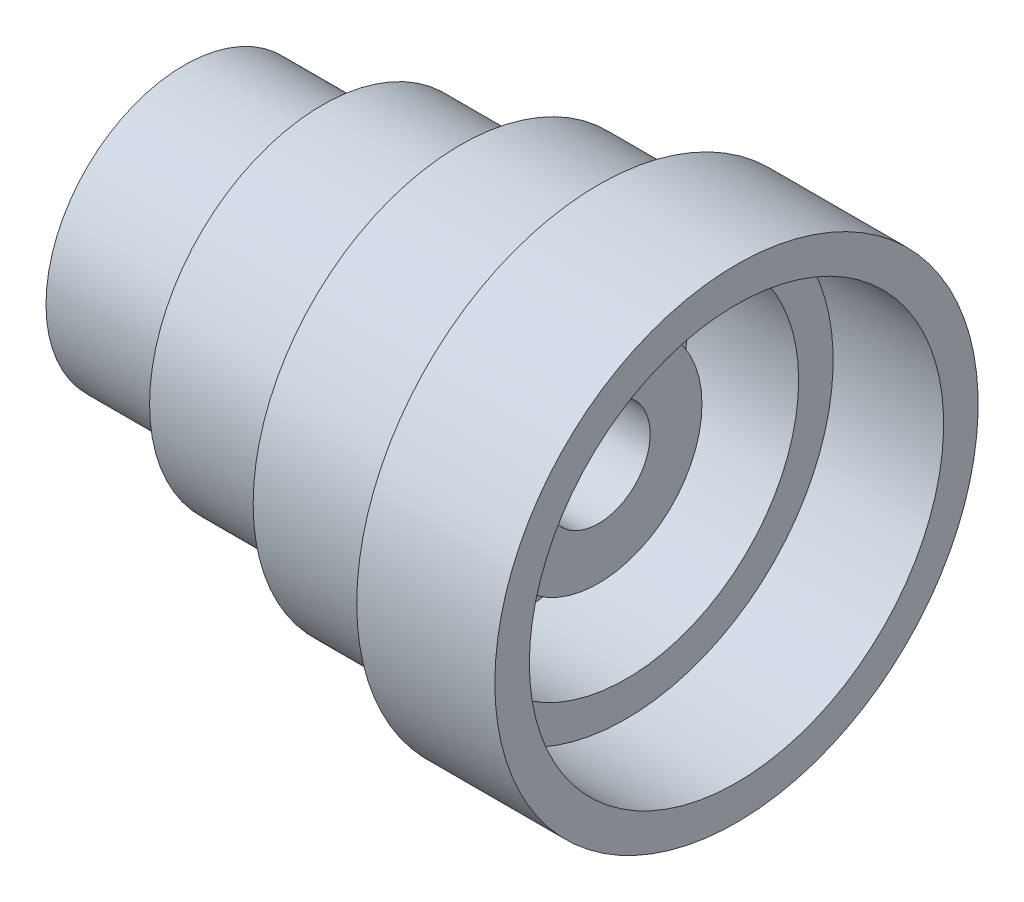
ISO-10303-21;
HEADER;
FILE_DESCRIPTION(('STEP AP214'),'2;1');
FILE_NAME('part.step','',(''),(''),'','','');
FILE_SCHEMA(('AUTOMOTIVE_DESIGN { 1 0 10303 214 1 1 1 1 }'));
ENDSEC;
DATA;
#1=APPLICATION_CONTEXT('core data for automotive mechanical design processes');
#2=APPLICATION_PROTOCOL_DEFINITION('international standard','automotive_design',2000,#1);
#3=PRODUCT_CONTEXT('',#1,'mechanical');
#4=PRODUCT('Part','Part','',(#3));
#5=PRODUCT_RELATED_PRODUCT_CATEGORY('part','',(#4));
#6=PRODUCT_DEFINITION_FORMATION('','',#4);
#7=PRODUCT_DEFINITION_CONTEXT('part definition',#1,'design');
#8=PRODUCT_DEFINITION('design','',#6,#7);
#9=PRODUCT_DEFINITION_SHAPE('','',#8);
#10=(LENGTH_UNIT() NAMED_UNIT(*) SI_UNIT(.MILLI.,.METRE.));
#11=(NAMED_UNIT(*) PLANE_ANGLE_UNIT() SI_UNIT($,.RADIAN.));
#12=(NAMED_UNIT(*) SI_UNIT($,.STERADIAN.) SOLID_ANGLE_UNIT());
#13=UNCERTAINTY_MEASURE_WITH_UNIT(LENGTH_MEASURE(1.E-05),#10,'distance_accuracy_value','');
#14=(GEOMETRIC_REPRESENTATION_CONTEXT(3) GLOBAL_UNCERTAINTY_ASSIGNED_CONTEXT((#13)) GLOBAL_UNIT_ASSIGNED_CONTEXT((#10,
#11,#12)) REPRESENTATION_CONTEXT('',''));
#15=CARTESIAN_POINT('',(0.,0.,0.));
#16=DIRECTION('',(0.,0.,1.));
#17=DIRECTION('',(1.,0.,0.));
#18=AXIS2_PLACEMENT_3D('',#15,#16,#17);
#19=CARTESIAN_POINT('',(-96.9856636191065,0.,0.));
#20=DIRECTION('',(-1.,0.,0.));
#21=DIRECTION('',(0.,0.,1.));
#22=AXIS2_PLACEMENT_3D('',#19,#20,#21);
#23=CYLINDRICAL_SURFACE('',#22,15.);
#24=CARTESIAN_POINT('',(77.592099478672,0.,0.));
#25=DIRECTION('',(-1.,0.,0.));
#26=DIRECTION('',(0.,0.,1.));
#27=AXIS2_PLACEMENT_3D('',#24,#25,#26);
#28=CIRCLE('',#27,15.);
#29=CARTESIAN_POINT('',(77.592099478672,0.,15.));
#30=VERTEX_POINT('',#29);
#31=EDGE_CURVE('E10',#30,#30,#28,.T.);
#32=ORIENTED_EDGE('',*,*,#31,.F.);
#33=EDGE_LOOP('',(#32));
#34=FACE_BOUND('',#33,.T.);
#35=CARTESIAN_POINT('',(-42.407900521328,0.,0.));
#36=DIRECTION('',(-1.,0.,0.));
#37=DIRECTION('',(0.,0.,1.));
#38=AXIS2_PLACEMENT_3D('',#35,#36,#37);
#39=CIRCLE('',#38,15.);
#40=CARTESIAN_POINT('',(-42.407900521328,0.,15.));
#41=VERTEX_POINT('',#40);
#42=EDGE_CURVE('E92',#41,#41,#39,.T.);
#43=ORIENTED_EDGE('',*,*,#42,.T.);
#44=EDGE_LOOP('',(#43));
#45=FACE_BOUND('',#44,.T.);
#46=ADVANCED_FACE('F40',(#34,#45),#23,.F.);
#47=CARTESIAN_POINT('',(77.592099478672,15.,0.));
#48=DIRECTION('',(-1.,0.,0.));
#49=DIRECTION('',(0.,0.,1.));
#50=AXIS2_PLACEMENT_3D('',#47,#48,#49);
#51=PLANE('',#50);
#52=CARTESIAN_POINT('',(77.592099478672,0.,0.));
#53=DIRECTION('',(-1.,0.,0.));
#54=DIRECTION('',(0.,0.,1.));
#55=AXIS2_PLACEMENT_3D('',#52,#53,#54);
#56=CIRCLE('',#55,30.);
#57=CARTESIAN_POINT('',(77.592099478672,0.,30.));
#58=VERTEX_POINT('',#57);
#59=EDGE_CURVE('E43',#58,#58,#56,.T.);
#60=ORIENTED_EDGE('',*,*,#59,.F.);
#61=EDGE_LOOP('',(#60));
#62=FACE_BOUND('',#61,.T.);
#63=ORIENTED_EDGE('',*,*,#31,.T.);
#64=EDGE_LOOP('',(#63));
#65=FACE_BOUND('',#64,.T.);
#66=ADVANCED_FACE('F195',(#62,#65),#51,.F.);
#67=CARTESIAN_POINT('',(-96.9856636191065,0.,0.));
#68=DIRECTION('',(-1.,0.,0.));
#69=DIRECTION('',(0.,0.,1.));
#70=AXIS2_PLACEMENT_3D('',#67,#68,#69);
#71=CYLINDRICAL_SURFACE('',#70,30.);
#72=CARTESIAN_POINT('',(21.592099478672,0.,0.));
#73=DIRECTION('',(-1.,0.,0.));
#74=DIRECTION('',(0.,0.,1.));
#75=AXIS2_PLACEMENT_3D('',#72,#73,#74);
#76=CIRCLE('',#75,30.);
#77=CARTESIAN_POINT('',(21.592099478672,0.,30.));
#78=VERTEX_POINT('',#77);
#79=EDGE_CURVE('E50',#78,#78,#76,.T.);
#80=ORIENTED_EDGE('',*,*,#79,.F.);
#81=EDGE_LOOP('',(#80));
#82=FACE_BOUND('',#81,.T.);
#83=ORIENTED_EDGE('',*,*,#59,.T.);
#84=EDGE_LOOP('',(#83));
#85=FACE_BOUND('',#84,.T.);
#86=ADVANCED_FACE('F190',(#82,#85),#71,.T.);
#87=CARTESIAN_POINT('',(21.592099478672,40.,0.));
#88=DIRECTION('',(-1.,0.,0.));
#89=DIRECTION('',(0.,0.,1.));
#90=AXIS2_PLACEMENT_3D('',#87,#88,#89);
#91=PLANE('',#90);
#92=CARTESIAN_POINT('',(21.592099478672,0.,0.));
#93=DIRECTION('',(-1.,0.,0.));
#94=DIRECTION('',(0.,0.,1.));
#95=AXIS2_PLACEMENT_3D('',#92,#93,#94);
#96=CIRCLE('',#95,40.);
#97=CARTESIAN_POINT('',(21.592099478672,0.,40.));
#98=VERTEX_POINT('',#97);
#99=EDGE_CURVE('E51',#98,#98,#96,.T.);
#100=ORIENTED_EDGE('',*,*,#99,.F.);
#101=EDGE_LOOP('',(#100));
#102=FACE_BOUND('',#101,.T.);
#103=ORIENTED_EDGE('',*,*,#79,.T.);
#104=EDGE_LOOP('',(#103));
#105=FACE_BOUND('',#104,.T.);
#106=ADVANCED_FACE('F182',(#102,#105),#91,.F.);
#107=CARTESIAN_POINT('',(-96.9856636191065,0.,0.));
#108=DIRECTION('',(-1.,0.,0.));
#109=DIRECTION('',(0.,0.,1.));
#110=AXIS2_PLACEMENT_3D('',#107,#108,#109);
#111=CYLINDRICAL_SURFACE('',#110,40.);
#112=CARTESIAN_POINT('',(53.592099478672,0.,0.));
#113=DIRECTION('',(-1.,0.,0.));
#114=DIRECTION('',(0.,0.,1.));
#115=AXIS2_PLACEMENT_3D('',#112,#113,#114);
#116=CIRCLE('',#115,40.);
#117=CARTESIAN_POINT('',(53.592099478672,0.,40.));
#118=VERTEX_POINT('',#117);
#119=EDGE_CURVE('E57',#118,#118,#116,.T.);
#120=ORIENTED_EDGE('',*,*,#119,.F.);
#121=EDGE_LOOP('',(#120));
#122=FACE_BOUND('',#121,.T.);
#123=ORIENTED_EDGE('',*,*,#99,.T.);
#124=EDGE_LOOP('',(#123));
#125=FACE_BOUND('',#124,.T.);
#126=ADVANCED_FACE('F173',(#122,#125),#111,.F.);
#127=CARTESIAN_POINT('',(53.592099478672,50.,0.));
#128=DIRECTION('',(-1.,0.,0.));
#129=DIRECTION('',(0.,0.,1.));
#130=AXIS2_PLACEMENT_3D('',#127,#128,#129);
#131=PLANE('',#130);
#132=CARTESIAN_POINT('',(53.592099478672,0.,0.));
#133=DIRECTION('',(-1.,0.,0.));
#134=DIRECTION('',(0.,0.,1.));
#135=AXIS2_PLACEMENT_3D('',#132,#133,#134);
#136=CIRCLE('',#135,50.);
#137=CARTESIAN_POINT('',(53.592099478672,0.,50.));
#138=VERTEX_POINT('',#137);
#139=EDGE_CURVE('E56',#138,#138,#136,.T.);
#140=ORIENTED_EDGE('',*,*,#139,.F.);
#141=EDGE_LOOP('',(#140));
#142=FACE_BOUND('',#141,.T.);
#143=ORIENTED_EDGE('',*,*,#119,.T.);
#144=EDGE_LOOP('',(#143));
#145=FACE_BOUND('',#144,.T.);
#146=ADVANCED_FACE('F166',(#142,#145),#131,.F.);
#147=CARTESIAN_POINT('',(-96.9856636191065,0.,0.));
#148=DIRECTION('',(-1.,0.,0.));
#149=DIRECTION('',(0.,0.,1.));
#150=AXIS2_PLACEMENT_3D('',#147,#148,#149);
#151=CYLINDRICAL_SURFACE('',#150,50.);
#152=CARTESIAN_POINT('',(85.592099478672,0.,0.));
#153=DIRECTION('',(-1.,0.,0.));
#154=DIRECTION('',(0.,0.,1.));
#155=AXIS2_PLACEMENT_3D('',#152,#153,#154);
#156=CIRCLE('',#155,50.);
#157=CARTESIAN_POINT('',(85.592099478672,0.,50.));
#158=VERTEX_POINT('',#157);
#159=EDGE_CURVE('E65',#158,#158,#156,.T.);
#160=ORIENTED_EDGE('',*,*,#159,.F.);
#161=EDGE_LOOP('',(#160));
#162=FACE_BOUND('',#161,.T.);
#163=ORIENTED_EDGE('',*,*,#139,.T.);
#164=EDGE_LOOP('',(#163));
#165=FACE_BOUND('',#164,.T.);
#166=ADVANCED_FACE('F162',(#162,#165),#151,.F.);
#167=CARTESIAN_POINT('',(85.592099478672,60.,0.));
#168=DIRECTION('',(-1.,0.,0.));
#169=DIRECTION('',(0.,0.,1.));
#170=AXIS2_PLACEMENT_3D('',#167,#168,#169);
#171=PLANE('',#170);
#172=CARTESIAN_POINT('',(85.592099478672,0.,0.));
#173=DIRECTION('',(-1.,0.,0.));
#174=DIRECTION('',(0.,0.,1.));
#175=AXIS2_PLACEMENT_3D('',#172,#173,#174);
#176=CIRCLE('',#175,60.);
#177=CARTESIAN_POINT('',(85.592099478672,0.,60.));
#178=VERTEX_POINT('',#177);
#179=EDGE_CURVE('E63',#178,#178,#176,.T.);
#180=ORIENTED_EDGE('',*,*,#179,.F.);
#181=EDGE_LOOP('',(#180));
#182=FACE_BOUND('',#181,.T.);
#183=ORIENTED_EDGE('',*,*,#159,.T.);
#184=EDGE_LOOP('',(#183));
#185=FACE_BOUND('',#184,.T.);
#186=ADVANCED_FACE('F160',(#182,#185),#171,.F.);
#187=CARTESIAN_POINT('',(-96.9856636191065,0.,0.));
#188=DIRECTION('',(-1.,0.,0.));
#189=DIRECTION('',(0.,0.,1.));
#190=AXIS2_PLACEMENT_3D('',#187,#188,#189);
#191=CYLINDRICAL_SURFACE('',#190,60.);
#192=CARTESIAN_POINT('',(117.592099478672,0.,0.));
#193=DIRECTION('',(-1.,0.,0.));
#194=DIRECTION('',(0.,0.,1.));
#195=AXIS2_PLACEMENT_3D('',#192,#193,#194);
#196=CIRCLE('',#195,60.);
#197=CARTESIAN_POINT('',(117.592099478672,0.,60.));
#198=VERTEX_POINT('',#197);
#199=EDGE_CURVE('E67',#198,#198,#196,.T.);
#200=ORIENTED_EDGE('',*,*,#199,.F.);
#201=EDGE_LOOP('',(#200));
#202=FACE_BOUND('',#201,.T.);
#203=ORIENTED_EDGE('',*,*,#179,.T.);
#204=EDGE_LOOP('',(#203));
#205=FACE_BOUND('',#204,.T.);
#206=ADVANCED_FACE('F151',(#202,#205),#191,.F.);
#207=CARTESIAN_POINT('',(117.592099478672,70.,0.));
#208=DIRECTION('',(-1.,0.,0.));
#209=DIRECTION('',(0.,0.,1.));
#210=AXIS2_PLACEMENT_3D('',#207,#208,#209);
#211=PLANE('',#210);
#212=CARTESIAN_POINT('',(117.592099478672,0.,0.));
#213=DIRECTION('',(-1.,0.,0.));
#214=DIRECTION('',(0.,0.,1.));
#215=AXIS2_PLACEMENT_3D('',#212,#213,#214);
#216=CIRCLE('',#215,70.);
#217=CARTESIAN_POINT('',(117.592099478672,0.,70.));
#218=VERTEX_POINT('',#217);
#219=EDGE_CURVE('E72',#218,#218,#216,.T.);
#220=ORIENTED_EDGE('',*,*,#219,.F.);
#221=EDGE_LOOP('',(#220));
#222=FACE_BOUND('',#221,.T.);
#223=ORIENTED_EDGE('',*,*,#199,.T.);
#224=EDGE_LOOP('',(#223));
#225=FACE_BOUND('',#224,.T.);
#226=ADVANCED_FACE('F144',(#222,#225),#211,.F.);
#227=CARTESIAN_POINT('',(-96.9856636191065,0.,0.));
#228=DIRECTION('',(-1.,0.,0.));
#229=DIRECTION('',(0.,0.,1.));
#230=AXIS2_PLACEMENT_3D('',#227,#228,#229);
#231=CYLINDRICAL_SURFACE('',#230,70.);
#232=CARTESIAN_POINT('',(77.592099478672,0.,0.));
#233=DIRECTION('',(-1.,0.,0.));
#234=DIRECTION('',(0.,0.,1.));
#235=AXIS2_PLACEMENT_3D('',#232,#233,#234);
#236=CIRCLE('',#235,70.);
#237=CARTESIAN_POINT('',(77.592099478672,0.,70.));
#238=VERTEX_POINT('',#237);
#239=EDGE_CURVE('E74',#238,#238,#236,.T.);
#240=ORIENTED_EDGE('',*,*,#239,.F.);
#241=EDGE_LOOP('',(#240));
#242=FACE_BOUND('',#241,.T.);
#243=ORIENTED_EDGE('',*,*,#219,.T.);
#244=EDGE_LOOP('',(#243));
#245=FACE_BOUND('',#244,.T.);
#246=ADVANCED_FACE('F138',(#242,#245),#231,.T.);
#247=CARTESIAN_POINT('',(77.592099478672,60.,0.));
#248=DIRECTION('',(1.,0.,0.));
#249=DIRECTION('',(0.,0.,-1.));
#250=AXIS2_PLACEMENT_3D('',#247,#248,#249);
#251=PLANE('',#250);
#252=CARTESIAN_POINT('',(77.592099478672,0.,0.));
#253=DIRECTION('',(-1.,0.,0.));
#254=DIRECTION('',(0.,0.,1.));
#255=AXIS2_PLACEMENT_3D('',#252,#253,#254);
#256=CIRCLE('',#255,60.);
#257=CARTESIAN_POINT('',(77.592099478672,0.,60.));
#258=VERTEX_POINT('',#257);
#259=EDGE_CURVE('E80',#258,#258,#256,.T.);
#260=ORIENTED_EDGE('',*,*,#259,.F.);
#261=EDGE_LOOP('',(#260));
#262=FACE_BOUND('',#261,.T.);
#263=ORIENTED_EDGE('',*,*,#239,.T.);
#264=EDGE_LOOP('',(#263));
#265=FACE_BOUND('',#264,.T.);
#266=ADVANCED_FACE('F134',(#262,#265),#251,.F.);
#267=CARTESIAN_POINT('',(-96.9856636191065,0.,0.));
#268=DIRECTION('',(-1.,0.,0.));
#269=DIRECTION('',(0.,0.,1.));
#270=AXIS2_PLACEMENT_3D('',#267,#268,#269);
#271=CYLINDRICAL_SURFACE('',#270,60.);
#272=CARTESIAN_POINT('',(37.592099478672,0.,0.));
#273=DIRECTION('',(-1.,0.,0.));
#274=DIRECTION('',(0.,0.,1.));
#275=AXIS2_PLACEMENT_3D('',#272,#273,#274);
#276=CIRCLE('',#275,60.);
#277=CARTESIAN_POINT('',(37.592099478672,0.,60.));
#278=VERTEX_POINT('',#277);
#279=EDGE_CURVE('E78',#278,#278,#276,.T.);
#280=ORIENTED_EDGE('',*,*,#279,.F.);
#281=EDGE_LOOP('',(#280));
#282=FACE_BOUND('',#281,.T.);
#283=ORIENTED_EDGE('',*,*,#259,.T.);
#284=EDGE_LOOP('',(#283));
#285=FACE_BOUND('',#284,.T.);
#286=ADVANCED_FACE('F130',(#282,#285),#271,.T.);
#287=CARTESIAN_POINT('',(37.592099478672,50.,0.));
#288=DIRECTION('',(1.,0.,0.));
#289=DIRECTION('',(0.,0.,-1.));
#290=AXIS2_PLACEMENT_3D('',#287,#288,#289);
#291=PLANE('',#290);
#292=CARTESIAN_POINT('',(37.592099478672,0.,0.));
#293=DIRECTION('',(-1.,0.,0.));
#294=DIRECTION('',(0.,0.,1.));
#295=AXIS2_PLACEMENT_3D('',#292,#293,#294);
#296=CIRCLE('',#295,50.);
#297=CARTESIAN_POINT('',(37.592099478672,0.,50.));
#298=VERTEX_POINT('',#297);
#299=EDGE_CURVE('E82',#298,#298,#296,.T.);
#300=ORIENTED_EDGE('',*,*,#299,.F.);
#301=EDGE_LOOP('',(#300));
#302=FACE_BOUND('',#301,.T.);
#303=ORIENTED_EDGE('',*,*,#279,.T.);
#304=EDGE_LOOP('',(#303));
#305=FACE_BOUND('',#304,.T.);
#306=ADVANCED_FACE('F121',(#302,#305),#291,.F.);
#307=CARTESIAN_POINT('',(-96.9856636191065,0.,0.));
#308=DIRECTION('',(-1.,0.,0.));
#309=DIRECTION('',(0.,0.,1.));
#310=AXIS2_PLACEMENT_3D('',#307,#308,#309);
#311=CYLINDRICAL_SURFACE('',#310,50.);
#312=CARTESIAN_POINT('',(-2.40790052132803,0.,0.));
#313=DIRECTION('',(-1.,0.,0.));
#314=DIRECTION('',(0.,0.,1.));
#315=AXIS2_PLACEMENT_3D('',#312,#313,#314);
#316=CIRCLE('',#315,50.);
#317=CARTESIAN_POINT('',(-2.40790052132803,0.,50.));
#318=VERTEX_POINT('',#317);
#319=EDGE_CURVE('E88',#318,#318,#316,.T.);
#320=ORIENTED_EDGE('',*,*,#319,.F.);
#321=EDGE_LOOP('',(#320));
#322=FACE_BOUND('',#321,.T.);
#323=ORIENTED_EDGE('',*,*,#299,.T.);
#324=EDGE_LOOP('',(#323));
#325=FACE_BOUND('',#324,.T.);
#326=ADVANCED_FACE('F113',(#322,#325),#311,.T.);
#327=CARTESIAN_POINT('',(-2.40790052132803,40.,0.));
#328=DIRECTION('',(1.,0.,0.));
#329=DIRECTION('',(0.,0.,-1.));
#330=AXIS2_PLACEMENT_3D('',#327,#328,#329);
#331=PLANE('',#330);
#332=CARTESIAN_POINT('',(-2.40790052132803,0.,0.));
#333=DIRECTION('',(-1.,0.,0.));
#334=DIRECTION('',(0.,0.,1.));
#335=AXIS2_PLACEMENT_3D('',#332,#333,#334);
#336=CIRCLE('',#335,40.);
#337=CARTESIAN_POINT('',(-2.40790052132803,0.,40.));
#338=VERTEX_POINT('',#337);
#339=EDGE_CURVE('E90',#338,#338,#336,.T.);
#340=ORIENTED_EDGE('',*,*,#339,.F.);
#341=EDGE_LOOP('',(#340));
#342=FACE_BOUND('',#341,.T.);
#343=ORIENTED_EDGE('',*,*,#319,.T.);
#344=EDGE_LOOP('',(#343));
#345=FACE_BOUND('',#344,.T.);
#346=ADVANCED_FACE('F108',(#342,#345),#331,.F.);
#347=CARTESIAN_POINT('',(-96.9856636191065,0.,0.));
#348=DIRECTION('',(-1.,0.,0.));
#349=DIRECTION('',(0.,0.,1.));
#350=AXIS2_PLACEMENT_3D('',#347,#348,#349);
#351=CYLINDRICAL_SURFACE('',#350,40.);
#352=CARTESIAN_POINT('',(-42.407900521328,0.,0.));
#353=DIRECTION('',(-1.,0.,0.));
#354=DIRECTION('',(0.,0.,1.));
#355=AXIS2_PLACEMENT_3D('',#352,#353,#354);
#356=CIRCLE('',#355,40.);
#357=CARTESIAN_POINT('',(-42.407900521328,0.,40.));
#358=VERTEX_POINT('',#357);
#359=EDGE_CURVE('E95',#358,#358,#356,.T.);
#360=ORIENTED_EDGE('',*,*,#359,.F.);
#361=EDGE_LOOP('',(#360));
#362=FACE_BOUND('',#361,.T.);
#363=ORIENTED_EDGE('',*,*,#339,.T.);
#364=EDGE_LOOP('',(#363));
#365=FACE_BOUND('',#364,.T.);
#366=ADVANCED_FACE('F103',(#362,#365),#351,.T.);
#367=CARTESIAN_POINT('',(-42.407900521328,15.,0.));
#368=DIRECTION('',(1.,0.,0.));
#369=DIRECTION('',(0.,0.,-1.));
#370=AXIS2_PLACEMENT_3D('',#367,#368,#369);
#371=PLANE('',#370);
#372=ORIENTED_EDGE('',*,*,#42,.F.);
#373=EDGE_LOOP('',(#372));
#374=FACE_BOUND('',#373,.T.);
#375=ORIENTED_EDGE('',*,*,#359,.T.);
#376=EDGE_LOOP('',(#375));
#377=FACE_BOUND('',#376,.T.);
#378=ADVANCED_FACE('F99',(#374,#377),#371,.F.);
#379=CLOSED_SHELL('',(#46,#66,#86,#106,#126,#146,#166,#186,#206,#226,#246,#266,#286,#306,#326,
#346,#366,#378));
#380=MANIFOLD_SOLID_BREP('B2',#379);
#381=ADVANCED_BREP_SHAPE_REPRESENTATION('',(#18,#380),#14);
#382=SHAPE_DEFINITION_REPRESENTATION(#9,#381);
ENDSEC;
END-ISO-10303-21;
